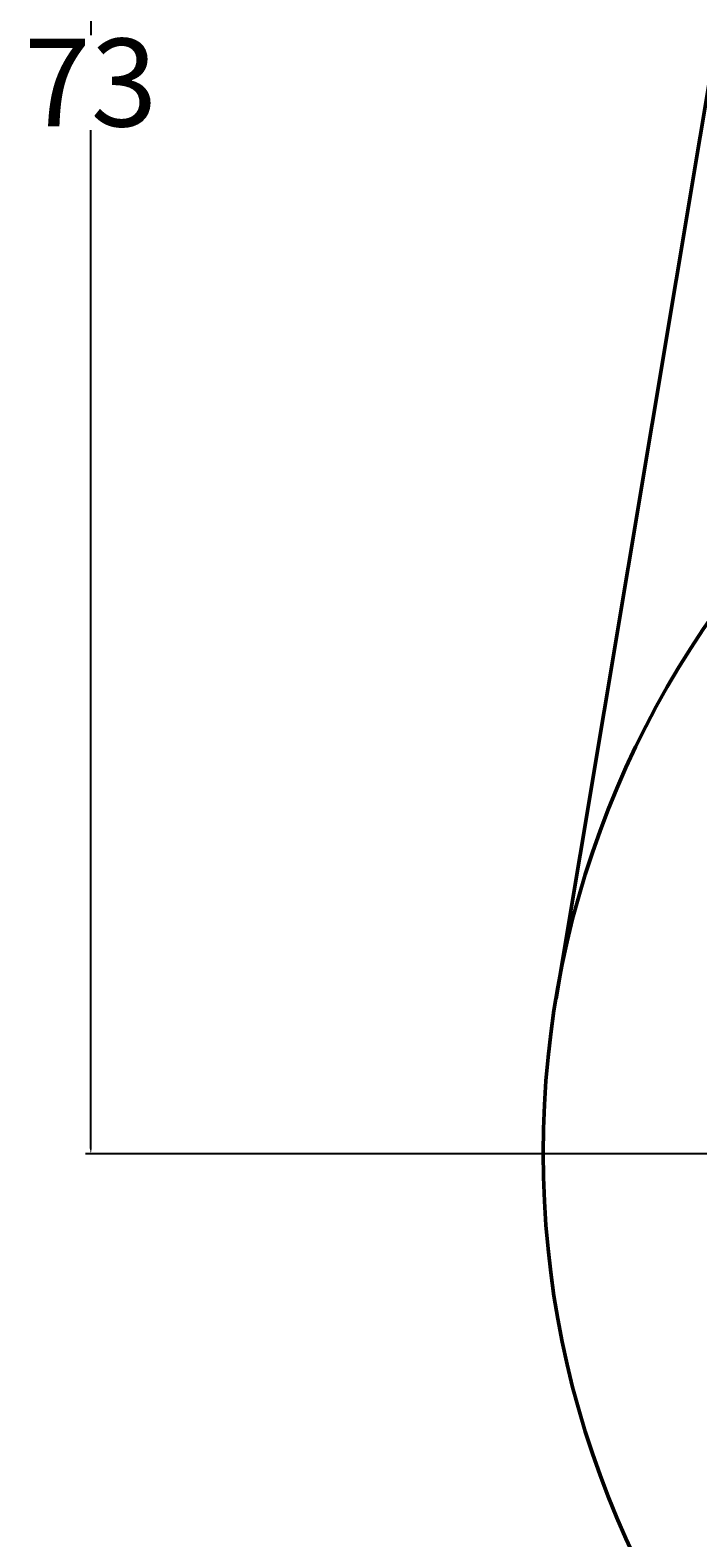
# Model space of a CAD drawing. Units: millimetres. Extents: x -50 to 109, y -46 to 152.
# Tile 2 of 18: x -50 to -28, y -20 to 32. Entities that reach past the tile are written whole.
import ezdxf

# ---------------------------------------------------------------- set-up
doc = ezdxf.new("R2010")
doc.units = ezdxf.units.MM
doc.header["$MEASUREMENT"] = 0
doc.layers.add('M-DIMS', color=2, linetype='Continuous', lineweight=25)
doc.layers.add('M-OUTL', color=7, linetype='Continuous', lineweight=50)
doc.styles.get("Standard").update_dxf_attribs({"font": 'arial.ttf'})
doc.dimstyles.get("Standard").update_dxf_attribs({"dimtxt": 0.18, "dimasz": 0.18, "dimexe": 0.18, "dimexo": 0.0625, "dimgap": 0.09, "dimtad": 0, "dimtih": 1, "dimtoh": 1, "dimdec": 4, "dimzin": 0, "dimdsep": 46, "dimtxsty": 'Standard', "dimcen": 0.09, "dimadec": 0, "dimazin": 0, "dimtfac": 1, "dimtdec": 4, "dimtofl": 0, "dimtmove": 0, "dimatfit": 3, "dimfxl": 1, "dimtolj": 1, "dimtzin": 0, "dimarcsym": 0})

# ---------------------------------------------------------------- blocks, each defined once
blk = doc.blocks.new('*D23')
at = {"layer": 'Defpoints', "color": 0, "transparency": 16777216}
for p in [(24.75, 12.317), (-26.598, -25.885)]:
    blk.add_point(p, dxfattribs=at)
at = {"layer": 'M-DIMS', "color": 0, "lineweight": -2, "transparency": 16777216}
for p, q in [((-0.924, -6.874), (-0.924, -6.694)), ((-1.014, -6.784), (-0.834, -6.784)), ((-30.604, -28.865), (-26.742, -25.992)), ((-30.784, -28.865), (-30.604, -28.865))]:
    blk.add_line(p, q, dxfattribs=at)
at = {"layer": 'M-DIMS', "color": 0, "transparency": 16777216}
blk.add_solid([(-26.76, -25.968), (-26.724, -26.016), (-26.598, -25.885)], dxfattribs=at)
at = {"layer": 'M-DIMS', "color": 0, "transparency": 16777216, "insert": (-34.648, -28.865), "char_height": 0.18, "attachment_point": 5}
blk.add_mtext('\\A1;{\\H16.66667x;%%C64}', dxfattribs=at)
blk = doc.blocks.new('*D25')
at = {"layer": 'Defpoints', "color": 0, "transparency": 16777216}
for p in [(0.007, 66.376), (-48.373, -6.811), (-0.299, -6.811)]:
    blk.add_point(p, dxfattribs=at)
at = {"layer": 'M-DIMS', "color": 0, "lineweight": -2, "transparency": 16777216}
for p, q in [((-0.056, 66.376), (-48.553, 66.376)), ((-48.373, 66.196), (-48.373, 31.405)), ((-48.373, -6.631), (-48.373, 28.16)), ((-0.361, -6.811), (-48.553, -6.811))]:
    blk.add_line(p, q, dxfattribs=at)
at = {"layer": 'M-DIMS', "color": 0, "transparency": 16777216}
for points in [[(-48.403, 66.196), (-48.343, 66.196), (-48.373, 66.376)], [(-48.403, -6.631), (-48.343, -6.631), (-48.373, -6.811)]]:
    blk.add_solid(points, dxfattribs=at)
at = {"layer": 'M-DIMS', "color": 0, "transparency": 16777216, "insert": (-48.373, 29.782), "char_height": 0.18, "attachment_point": 5}
blk.add_mtext('\\A1;{\\H16.66667x;73}', dxfattribs=at)
blk = doc.blocks.new('*D29')
at = {"layer": 'Defpoints', "color": 0, "transparency": 16777216}
for p in [(21.684, 15.863), (-23.531, -29.431)]:
    blk.add_point(p, dxfattribs=at)
at = {"layer": 'M-DIMS', "color": 0, "lineweight": -2, "transparency": 16777216}
for p, q in [((-0.924, -6.874), (-0.924, -6.694)), ((-1.014, -6.784), (-0.834, -6.784)), ((-37.096, -43.02), (-23.658, -29.559)), ((-37.276, -43.02), (-37.096, -43.02))]:
    blk.add_line(p, q, dxfattribs=at)
at = {"layer": 'M-DIMS', "color": 0, "transparency": 16777216}
blk.add_solid([(-23.68, -29.537), (-23.637, -29.58), (-23.531, -29.431)], dxfattribs=at)
at = {"layer": 'M-DIMS', "color": 0, "transparency": 16777216, "insert": (-37.592, -43.02), "char_height": 0.18, "attachment_point": 5}
blk.add_mtext('\\A1;∅64', dxfattribs=at)

msp = doc.modelspace()

# ---------------------------------------------------------------- linework, layer by layer
at = {"layer": 'M-OUTL'}
msp.add_line((-20.5811, 69.65018), (-32.48503, -1.5038), dxfattribs=at)
msp.add_circle((-0.92366, -6.78396), 32, dxfattribs=at)

# ---------------------------------------------------------------- dimensions: what is measured, and where the dimension line sits
at = {"layer": 'M-DIMS'}
dim = msp.add_linear_dim(base=(-48.37276, -6.81116), p1=(0.00669, 66.37611), p2=(-0.2986, -6.81116), angle=90, text='{\\H16.66667x;73}', dimstyle='Standard', override={"dimclrd": 0, "dimclre": 0, "dimclrt": 0}, dxfattribs=at)
dim.commit()
dim.dimension.update_dxf_attribs({"geometry": '*D25', "text_midpoint": (-48.37276, 29.78248)})
dim = msp.add_diameter_dim_2p(p1=(21.68387, 15.86332), p2=(-23.53119, -29.43125), dimstyle='Standard', override={"dimdec": 0, "dimlfac": 1, "dimrnd": 0, "dimzin": 0, "dimdsep": 46, "dimlunit": 2}, dxfattribs=at)
dim.commit()
dim.dimension.update_dxf_attribs({"geometry": '*D29', "text_midpoint": (-37.59218, -43.01962), "dimtype": 163})
dim = msp.add_diameter_dim_2p(p1=(24.75033, 12.31698), p2=(-26.59765, -25.88491), text='{\\H16.66667x;%%C64}', dimstyle='Standard', override={"dimclrd": 0, "dimclre": 0, "dimclrt": 0}, dxfattribs=at)
dim.commit()
dim.dimension.update_dxf_attribs({"geometry": '*D23', "text_midpoint": (-34.64806, -28.86518), "dimtype": 163})

doc.saveas('drawing.dxf')
